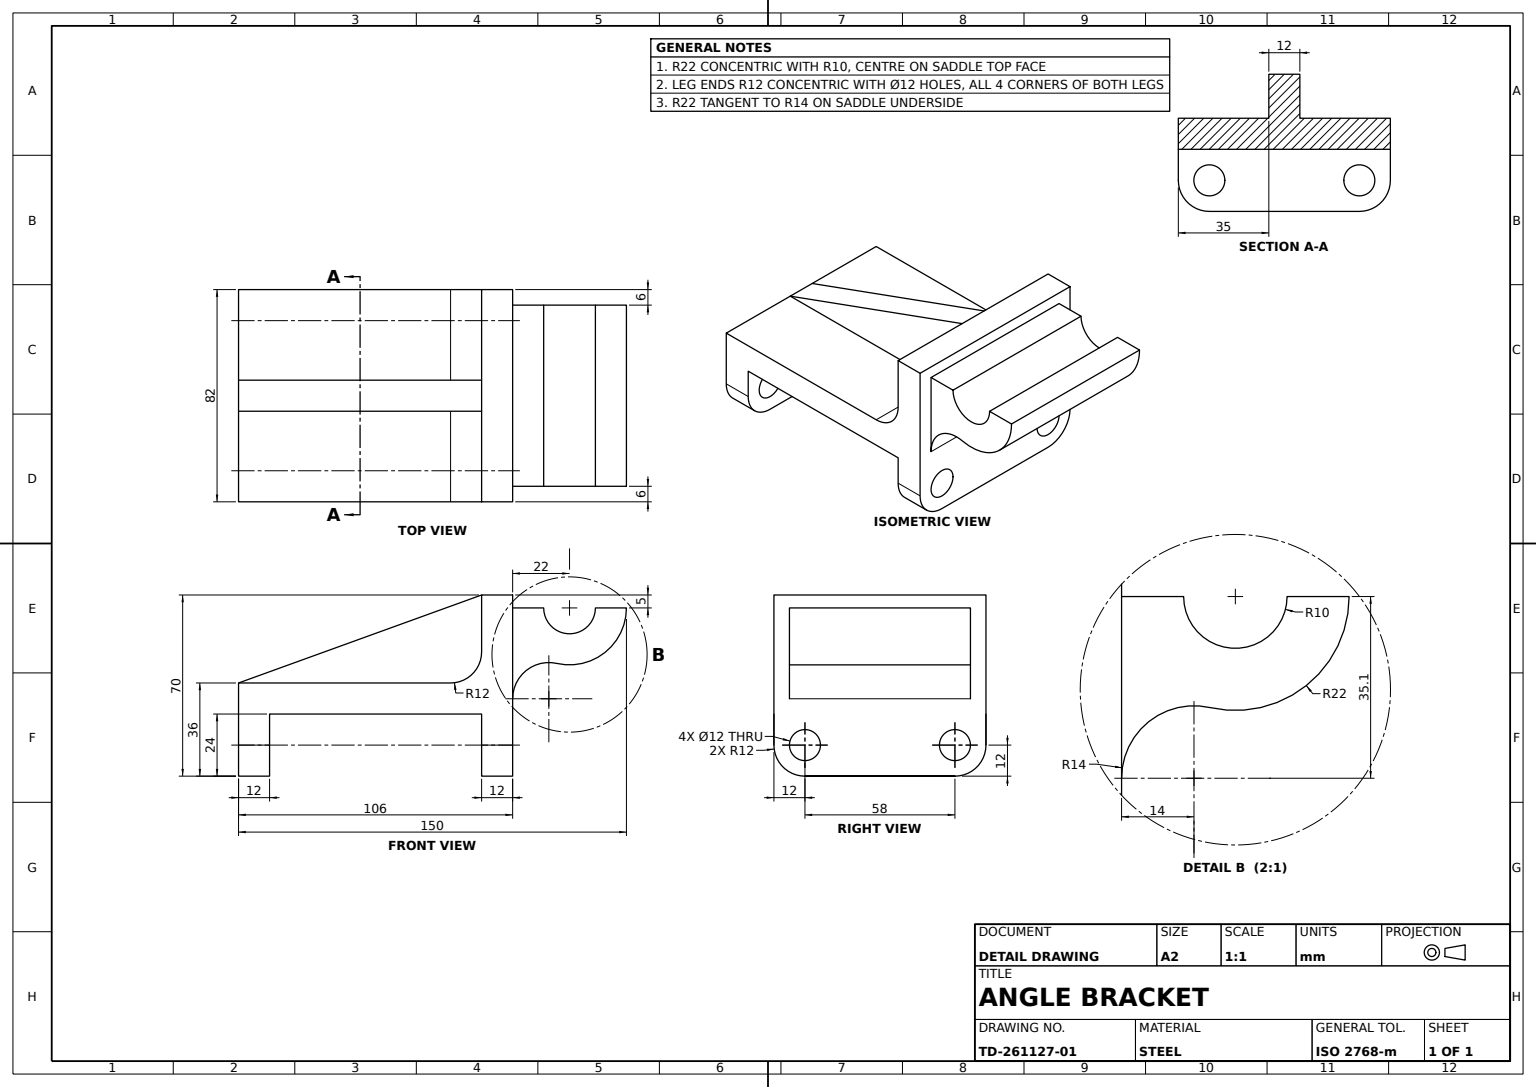
from build123d import *

# Parameters (mm, degrees)
BASE_PROFILE_SKETCH_W         = 106
BASE_PROFILE_SKETCH_H         = 82
BASE_BLOCK_DEPTH              = 36
UNDERSIDE_CHANNEL_SKETCH_W    = 82
UNDERSIDE_CHANNEL_SKETCH_H    = 24
UNDERSIDE_CHANNEL_CUT_DEPTH   = 105.062481231
BASE_CORNER_FILLETS_R12_R     = 12
MOUNTING_HOLES_SKETCH_R       = 6
MOUNTING_HOLES_12_DEPTH       = 120.218287188
UPRIGHT_PLATE_SKETCH_W        = 12
UPRIGHT_PLATE_SKETCH_H        = 34
UPRIGHT_PLATE_DEPTH           = 82
SADDLE_BLOCK_DEPTH            = 70
SADDLE_GROOVE_SKETCH_R        = 10
SADDLE_GROOVE_20_DEPTH        = 82
REINFORCING_RIB_REACH         = 128.452
REINFORCING_RIB_SKETCH_WALL_W = 354.863135512
REINFORCING_RIB_SKETCH_WALL_H = 12
UPRIGHT_PLATE_FILLETS_R12_R   = 12


with BuildPart() as part:
    # Base Profile Sketch → Base Block (new body)
    with BuildSketch(Plane(origin=(0, 0, 0), x_dir=(1, 0, 0), z_dir=(0, 1, 0))):
        Rectangle(BASE_PROFILE_SKETCH_W, BASE_PROFILE_SKETCH_H)
    extrude(amount=BASE_BLOCK_DEPTH)

    # Underside Channel Sketch → Underside Channel Cut (cut, through all)
    with BuildSketch(Plane.XY.offset(41)):
        with Locations((0, 12)):
            Rectangle(UNDERSIDE_CHANNEL_SKETCH_W, UNDERSIDE_CHANNEL_SKETCH_H)
    extrude(amount=-UNDERSIDE_CHANNEL_CUT_DEPTH, mode=Mode.SUBTRACT)

    # Base Corner Fillets R12
    base_corner_fillets_r12_edges = [part.edges().sort_by_distance(p)[0] for p in [
        (47, 0, 41),
        (-47, 0, -41),
        (-47, 0, 41),
        (47, 0, -41),
    ]]
    fillet(base_corner_fillets_r12_edges, radius=BASE_CORNER_FILLETS_R12_R)

    # Mounting Holes Sketch → Mounting Holes Ø12 (cut, through all)
    with BuildSketch(Plane.ZY.offset(53)):
        with Locations((29, 12)):
            Circle(MOUNTING_HOLES_SKETCH_R)
        with Locations((-29, 12)):
            Circle(MOUNTING_HOLES_SKETCH_R)
    extrude(amount=-MOUNTING_HOLES_12_DEPTH, mode=Mode.SUBTRACT)

    # Upright Plate Sketch → Upright Plate (add)
    with BuildSketch(Plane.XY.offset(41)):
        with Locations((47, 53)):
            Rectangle(UPRIGHT_PLATE_SKETCH_W, UPRIGHT_PLATE_SKETCH_H)
    extrude(amount=-UPRIGHT_PLATE_DEPTH)

    # Saddle Block Sketch → Saddle Block (add)
    with BuildSketch(Plane.XY.offset(35)):
        with BuildLine():
            Line((53, 65), (97, 65))
            ThreePointArc((97, 65), (88.719410418, 47.801808881), (70.111111111, 43.550087053))
            ThreePointArc((70.111111111, 43.550087053), (58.269466098, 40.84444589), (53, 29.90014245))
            Line((53, 29.90014245), (53, 65))
        make_face()
    extrude(amount=-SADDLE_BLOCK_DEPTH)

    # Saddle Groove Sketch → Saddle Groove Ø20 (cut)
    with BuildSketch(Plane.XY.offset(35)):
        with Locations((75, 65)):
            Circle(SADDLE_GROOVE_SKETCH_R)
    extrude(amount=-SADDLE_GROOVE_20_DEPTH, mode=Mode.SUBTRACT)

    # Reinforcing Rib Sketch wall → Reinforcing Rib (add, up to next)
    with BuildSketch(Plane(origin=(-6, 53, 0), x_dir=(-0.940376225751, -0.340136081654, 0), z_dir=(0.340136081654, -0.940376225751, 0)), mode=Mode.PRIVATE) as reinforcing_rib_sk1:
        Rectangle(REINFORCING_RIB_SKETCH_WALL_W, REINFORCING_RIB_SKETCH_WALL_H)
    reinforcing_rib_tool1 = extrude(reinforcing_rib_sk1.sketch, amount=REINFORCING_RIB_REACH, mode=Mode.PRIVATE) - part.part
    add(reinforcing_rib_tool1.solids().sort_by_distance((-6, 53, 0))[0])

    # Upright Plate Fillets R12
    upright_plate_fillets_r12_edges = [part.edges().sort_by_distance(p)[0] for p in [
        (41, 36, 23.5),
        (41, 36, -23.5),
    ]]
    fillet(upright_plate_fillets_r12_edges, radius=UPRIGHT_PLATE_FILLETS_R12_R)


solid = part.part
